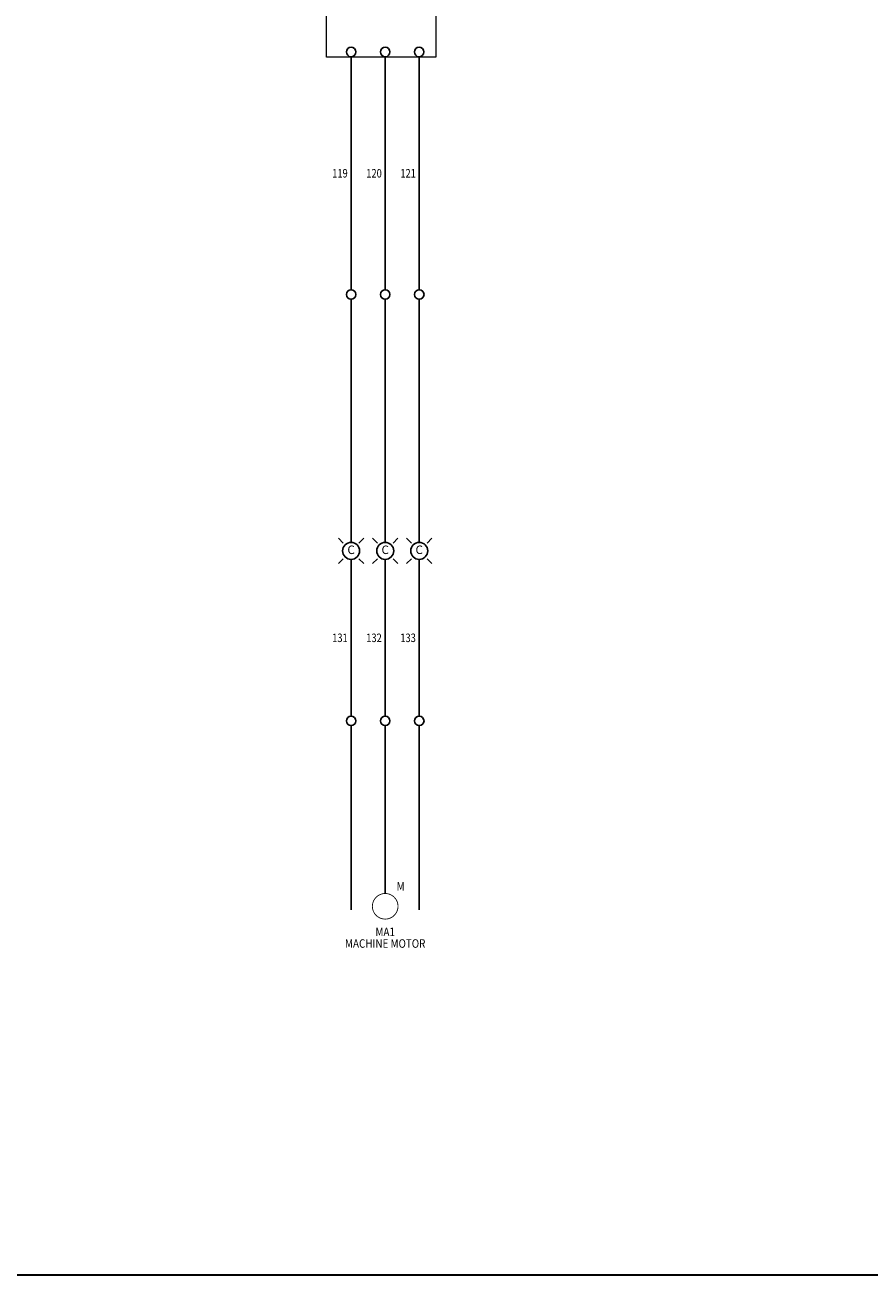
# Model space of a CAD drawing. Units: inches. Extents: x 12.5 to 62, y 4.7 to 37.4.
# Tile 2 of 5: x 24.9 to 37.3, y 4.7 to 23.1. Entities that reach past the tile are written whole.
import ezdxf
from ezdxf.enums import TextEntityAlignment as Align

# ---------------------------------------------------------------- set-up
doc = ezdxf.new("R2010")
doc.units = ezdxf.units.IN
doc.header["$MEASUREMENT"] = 0
for name, color, linetype, lineweight in [('16AWG-BLU', 182, 'Continuous', 25), ('16AWG-GRNYEL', 60, 'Continuous', 25), ('16AWG-RED', 1, 'Continuous', 25), ('E-ANNO-TTLB', 7, 'Continuous', 35), ('LOCBOX', 7, 'Continuous', 18), ('SYMS', 7, 'Continuous', 25), ('WIRENO', 72, 'Continuous', 18)]:
    doc.layers.add(name, color=color, linetype=linetype, lineweight=lineweight)
for name, color, linetype in [('DESC', 150, 'Continuous'), ('LOC', 8, 'Continuous'), ('MISC', 7, 'Continuous'), ('TAGS', 150, 'Continuous')]:
    doc.layers.add(name, color=color, linetype=linetype)
doc.styles.add('WD', font='romans.shx')

# ---------------------------------------------------------------- blocks, each defined once
blk = doc.blocks.new('VMO13_1-')
at = {"const_width": 0.0125}
blk.add_lwpolyline([(0, 0.188, 1), (0, -0.188, 1)], format="xyb", close=True, dxfattribs=at)
at = {"style": 'WD', "width": 0.85}
for tag, p in [('INST', (0.168, 0.402)), ('LOC', (0.168, 0.233))]:
    blk.add_attdef(tag, p, '', height=0.125, dxfattribs=at)
at = {"style": 'WD', "width": 0.85, "flags": 8}
blk.add_attdef('TERM01', text='', height=0.125, dxfattribs=at).set_placement((-0.064, 0.235), align=Align.RIGHT)
at = {"style": 'WD', "flags": 9}
blk.add_attdef('WDBLKNAM', text='', height=0.01, dxfattribs=at).set_placement((-0.056, 0.2), align=Align.RIGHT)
at = {"style": 'WD', "flags": 1}
blk.add_attdef('X2TERM01', (0, 0.188), '', height=0.0125, dxfattribs=at)
at = {"style": 'WD'}
for tag, height, width, p in [('RATING1', 0.1, 0.8, (0, 0)), ('TAG1', 0.125, 0.85, (0, -0.438)), ('DESC1', 0.125, 0.85, (0, -0.609)), ('DESC2', 0.125, 0.85, (0, -0.781)), ('DESC3', 0.125, 0.85, (0, -0.944)), ('RATING3', 0.125, 0.85, (0, -1.106)), ('RATING4', 0.125, 0.85, (0, -1.269)), ('WDTAGALT', 0.125, 0.85, (0, -1.431))]:
    blk.add_attdef(tag, text='', height=height, dxfattribs=dict(at, width=width)).set_placement(p, align=Align.CENTER)
at = {"style": 'WD', "flags": 9}
for tag, p in [('ASSYCODE', (0, 0.125)), ('FAMILY', (-0.005, 0.17)), ('WDTYPE', (0.004, 0.087))]:
    blk.add_attdef(tag, text='', height=0.01, dxfattribs=at).set_placement(p, align=Align.CENTER)
at = {"style": 'WD', "flags": 1}
for tag, p in [('MFG', (0, 0.14)), ('CAT', (0, 0.159))]:
    blk.add_attdef(tag, text='', height=0.01, dxfattribs=at).set_placement(p, align=Align.MIDDLE)
at = {"style": 'WD', "width": 0.8}
blk.add_attdef('RATING2', text='', height=0.1, dxfattribs=at).set_placement((0, -0.031), align=Align.TOP_CENTER)
blk = doc.blocks.new('VLT1C')
for p, q in [((-0.115, 0.115), (-0.186, 0.186)), ((0.115, 0.115), (0.186, 0.186)), ((-0.115, -0.115), (-0.186, -0.186)), ((0.115, -0.115), (0.186, -0.186))]:
    blk.add_line(p, q)
blk.add_circle((0, 0), 0.125)
at = {"style": 'WD'}
for tag, height, flags, p in [('TERM01', 0.125, 8, (-0.031, 0.219)), ('FAMILY', 0.01, 9, (-0.219, -0.117)), ('MFG', 0.01, 9, (-0.221, -0.149)), ('CAT', 0.01, 9, (-0.221, -0.134))]:
    blk.add_attdef(tag, text='', height=height, dxfattribs=dict(at, flags=flags)).set_placement(p, align=Align.RIGHT)
blk.add_attdef('COLOR', text='', height=0.125, dxfattribs=at).set_placement((0, 0), align=Align.MIDDLE)
at = {"style": 'WD', "flags": 1}
for tag, p in [('X2TERM01', (0, 0.125)), ('X8TERM02', (0, -0.125))]:
    blk.add_attdef(tag, p, '', height=0.0125, dxfattribs=at)
at = {"style": 'WD'}
for tag, p, width in [('TAG1', (0.2, -0.098), 0.9), ('DESC1', (-0.256, -0.931), 0.9), ('WDTAGALT', (-0.25, -1.25), 0.7)]:
    blk.add_attdef(tag, p, '', height=0.125, dxfattribs=dict(at, width=width))
at = {"style": 'WD', "flags": 9}
blk.add_attdef('ASSYCODE', text='', height=0.01, dxfattribs=at).set_placement((-0.238, -0.097), align=Align.CENTER)
at = {"style": 'WD'}
for tag, width, p in [('INST', 0.7, (0.281, -0.147)), ('LOC', 0.7, (0.281, -0.317)), ('DESC2', 0.9, (-0.256, -0.963))]:
    blk.add_attdef(tag, text='', height=0.125, dxfattribs=dict(at, width=width)).set_placement(p, align=Align.TOP_LEFT)
at = {"style": 'WD', "flags": 8}
blk.add_attdef('TERM02', text='', height=0.125, dxfattribs=at).set_placement((-0.031, -0.219), align=Align.TOP_RIGHT)
blk = doc.blocks.new('VT0_02')
blk.add_circle((0, 0), 0.0699)
at = {"style": 'WD', "flags": 1}
for tag, p in [('X4TERM01', (-0.07, 0)), ('X2TERM01', (0, 0.07)), ('X1TERM01', (0.07, 0)), ('X8TERM01', (0, -0.07))]:
    blk.add_attdef(tag, p, '', height=0.01, dxfattribs=at)
blk = doc.blocks.new('WD_WNV')
at = {"style": 'WD', "width": 0.8}
blk.add_attdef('WIRENO', text='', height=0.125, dxfattribs=at).set_placement((-0.05, 0), align=Align.MIDDLE_RIGHT)
at = {"style": 'WD', "flags": 1}
for tag, p in [('W01USER', (-0.062, 0.094)), ('W02USER', (-0.062, 0.086)), ('W03USER', (-0.062, 0.078)), ('W04USER', (-0.062, 0.07)), ('W05USER', (-0.062, 0.062)), ('W06USER', (-0.062, 0.055)), ('W07USER', (-0.062, 0.047)), ('W08USER', (-0.062, 0.039)), ('W09USER', (-0.062, 0.031)), ('W10USER', (-0.062, 0.023))]:
    blk.add_attdef(tag, text='', height=0.005, dxfattribs=at).set_placement(p, align=Align.CENTER)

msp = doc.modelspace()

# ---------------------------------------------------------------- linework, layer by layer
at = {"layer": '16AWG-BLU'}
for p, q in [((30.719, 22.637), (30.719, 19.214)), ((30.719, 19.074), (30.719, 15.503)), ((30.719, 15.253), (30.719, 12.95)), ((30.719, 12.811), (30.719, 10.104))]:
    msp.add_line(p, q, dxfattribs=at)
at = {"layer": '16AWG-GRNYEL'}
for p, q in [((30.219, 22.637), (30.219, 19.214)), ((30.219, 19.074), (30.219, 15.503)), ((30.219, 15.253), (30.219, 12.95)), ((30.219, 12.811), (30.219, 10.344))]:
    msp.add_line(p, q, dxfattribs=at)
at = {"layer": '16AWG-RED'}
for p, q in [((29.719, 22.637), (29.719, 19.214)), ((29.719, 19.074), (29.719, 15.503)), ((29.719, 15.253), (29.719, 12.95)), ((29.719, 12.811), (29.719, 10.104))]:
    msp.add_line(p, q, dxfattribs=at)
at = {"layer": 'E-ANNO-TTLB'}
msp.add_lwpolyline([(12.524, 37.377), (62.033, 37.377), (62.033, 4.741), (12.524, 4.741)], close=True, dxfattribs=at)
at = {"layer": 'LOCBOX'}
msp.add_lwpolyline([(29.357, 23.701), (30.964, 23.701), (30.964, 22.632), (29.357, 22.632)], close=True, dxfattribs=at)

# ---------------------------------------------------------------- block references
at = {"layer": 'SYMS'}
for p in [(29.719, 22.707), (30.219, 22.707), (30.717, 22.707), (29.719, 19.144), (30.219, 19.144), (30.719, 19.144), (29.719, 12.881), (30.219, 12.881), (30.719, 12.881)]:
    msp.add_blockref('VT0_02', p, dxfattribs=at)
ref = msp.add_blockref('VLT1C', (29.719, 15.378), dxfattribs=at)
ref.add_attrib('COLOR', 'C', dxfattribs={"layer": 'MISC', "height": 0.125, "style": 'WD'}).set_placement((29.719, 15.378), align=Align.MIDDLE)
ref = msp.add_blockref('VLT1C', (30.219, 15.378), dxfattribs=at)
ref.add_attrib('COLOR', 'C', dxfattribs={"layer": 'MISC', "height": 0.125, "style": 'WD'}).set_placement((30.219, 15.378), align=Align.MIDDLE)
ref = msp.add_blockref('VLT1C', (30.719, 15.378), dxfattribs=at)
ref.add_attrib('COLOR', 'C', dxfattribs={"layer": 'MISC', "height": 0.125, "style": 'WD'}).set_placement((30.719, 15.378), align=Align.MIDDLE)
ref = msp.add_blockref('VMO13_1-', (30.219, 10.157), dxfattribs=at)
ref.add_attrib('DESC1', 'MACHINE MOTOR', dxfattribs={"layer": 'DESC', "height": 0.125, "style": 'WD', "width": 0.85}).set_placement((30.219, 9.548), align=Align.CENTER)
ref.add_attrib('LOC', 'M', (30.387, 10.389), dxfattribs={"layer": 'LOC', "height": 0.125, "style": 'WD', "width": 0.85})
ref.add_attrib('TAG1', 'MA1', dxfattribs={"layer": 'TAGS', "height": 0.125, "style": 'WD', "width": 0.85}).set_placement((30.219, 9.719), align=Align.CENTER)
at = {"layer": 'WIRENO'}
ref = msp.add_blockref('WD_WNV', (29.719, 20.925), dxfattribs=at)
ref.add_attrib('WIRENO', '119', dxfattribs={"linetype": 'Continuous', "height": 0.125, "style": 'WD', "width": 0.8}).set_placement((29.669, 20.925), align=Align.MIDDLE_RIGHT)
ref = msp.add_blockref('WD_WNV', (30.219, 20.925), dxfattribs=at)
ref.add_attrib('WIRENO', '120', dxfattribs={"linetype": 'Continuous', "height": 0.125, "style": 'WD', "width": 0.8}).set_placement((30.169, 20.925), align=Align.MIDDLE_RIGHT)
ref = msp.add_blockref('WD_WNV', (30.719, 20.925), dxfattribs=at)
ref.add_attrib('WIRENO', '121', dxfattribs={"linetype": 'Continuous', "height": 0.125, "style": 'WD', "width": 0.8}).set_placement((30.669, 20.925), align=Align.MIDDLE_RIGHT)
ref = msp.add_blockref('WD_WNV', (29.719, 14.101), dxfattribs=at)
ref.add_attrib('WIRENO', '131', dxfattribs={"linetype": 'Continuous', "height": 0.125, "style": 'WD', "width": 0.8}).set_placement((29.669, 14.101), align=Align.MIDDLE_RIGHT)
ref = msp.add_blockref('WD_WNV', (30.219, 14.101), dxfattribs=at)
ref.add_attrib('WIRENO', '132', dxfattribs={"linetype": 'Continuous', "height": 0.125, "style": 'WD', "width": 0.8}).set_placement((30.169, 14.101), align=Align.MIDDLE_RIGHT)
ref = msp.add_blockref('WD_WNV', (30.719, 14.101), dxfattribs=at)
ref.add_attrib('WIRENO', '133', dxfattribs={"linetype": 'Continuous', "height": 0.125, "style": 'WD', "width": 0.8}).set_placement((30.669, 14.101), align=Align.MIDDLE_RIGHT)

doc.saveas('drawing.dxf')
